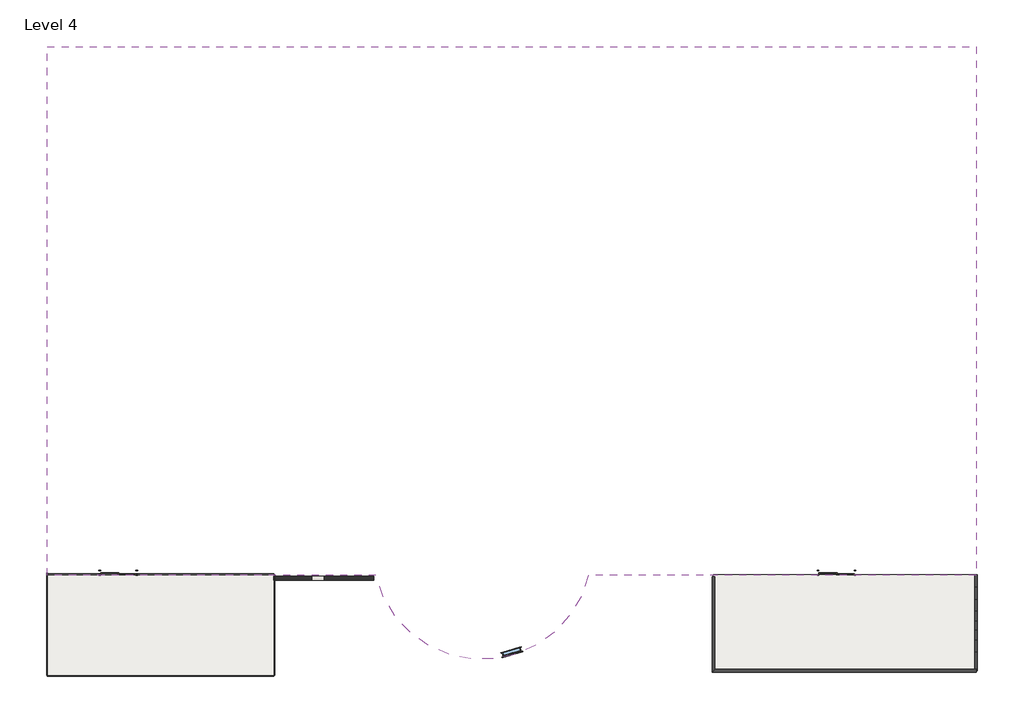
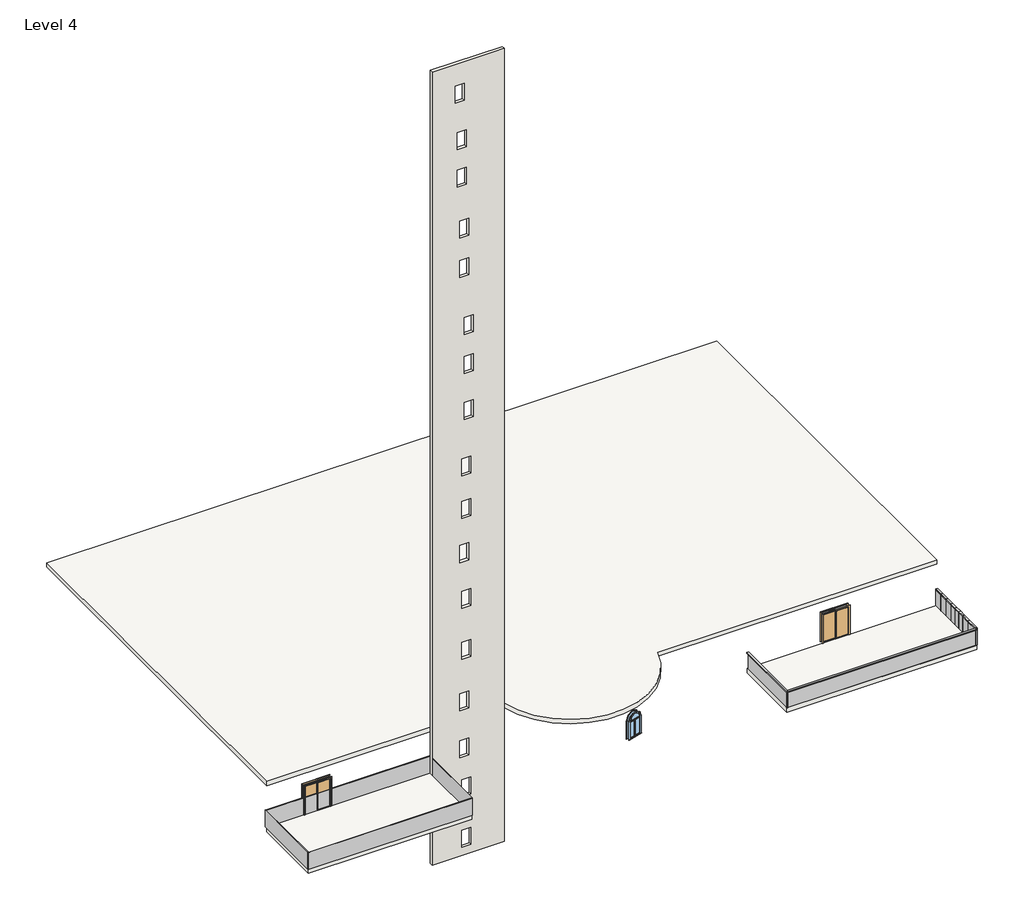
# One storey: 14 plates, 11 members, 3 slabs, 2 doors, 1 wall, 1 window.
"""IFC4 building model written with IfcOpenShell, lengths in millimetres."""

from ifc_helpers import new_model, si_unit, point, frame, frame_2d, origin, place, context, project, spatial, polyline, circle_curve, trimmed, segment, composite_curve, outline, extrude, transform, mapped, element, save
from components import door_076b30e0, member_75074519, member_47bfaf8a, member_15823cb3, member_e44847c7, member_d2e7e466, member_2fad0b47, member_fc190105, system_panel_glazed_7af1c9c3, system_panel_glazed_a18a7e0a, system_panel_glazed_7cd9bc56, system_panel_glazed_88916357, system_panel_glazed_11b37e3b, system_panel_glazed_6b3781c5, system_panel_glazed_3a47dc32, system_panel_glazed_b96adab1, system_panel_glazed_dcca9b78, window_cf4adaea

model = new_model("IFC4")

# Units and contexts
model_context = context("Model", 3, world=origin())
ifc_project = project(units=[si_unit("LENGTHUNIT", "METRE", prefix="MILLI")], contexts=[model_context])

# Site, building, storey
site = spatial("IfcSite", under=ifc_project)
building = spatial("IfcBuilding", under=site)
storey = spatial("IfcBuildingStorey", under=building, Name="Level 4", Elevation=6400.8)

# Doors
placement = place(None, origin())
door_shape = door_076b30e0(model_context)
element("IfcDoor", 1, ObjectType="Door-Double-Sliding : 68\" x 80\"", at=placement, inside=storey, context=model_context, shape_type="MappedRepresentation", body=[
    mapped(door_shape, transform((-16369.385279, -12227.7237084, 6400.8), x_axis=(-1.0, 0.0, 0.0), y_axis=(0.0, -1.0, 0.0), z_axis=(0.0, 0.0, 1.0))),
])
element("IfcDoor", 2, ObjectType="Door-Double-Sliding : 68\" x 80\"", at=placement, inside=storey, context=model_context, shape_type="MappedRepresentation", body=[
    mapped(door_shape, transform((18682.614721, -12227.7237084, 6400.8), x_axis=(-1.0, 0.0, 0.0), y_axis=(0.0, -1.0, 0.0), z_axis=(0.0, 0.0, 1.0))),
])

# Members
member_shape = member_75074519(model_context)
element("IfcMember", 3, ObjectType="Rectangular Mullion : 2.5\" x 5\" rectangular", at=placement, inside=storey, context=model_context, shape_type="MappedRepresentation", body=[
    mapped(member_shape, transform((25489.814721, -17133.9605259, 7620.0), x_axis=(0.0, -1.0, 0.0), y_axis=(1.0, 0.0, 0.0), z_axis=(0.0, 0.0, 1.0))),
])
member_2_shape = member_47bfaf8a(model_context)
element("IfcMember", 4, ObjectType="Rectangular Mullion : 2.5\" x 5\" rectangular", at=placement, inside=storey, context=model_context, shape_type="MappedRepresentation", body=[
    mapped(member_2_shape, transform((25489.814721, -15609.9605259, 7620.0), x_axis=(0.0, 0.0, 1.0), y_axis=(1.0, 0.0, 0.0), z_axis=(0.0, 1.0, 0.0))),
])
member_3_shape = member_15823cb3(model_context)
element("IfcMember", 5, ObjectType="Rectangular Mullion : 2.5\" x 5\" rectangular", at=placement, inside=storey, context=model_context, shape_type="MappedRepresentation", body=[
    mapped(member_3_shape, transform((25489.814721, -14238.3605259, 7620.0), x_axis=(0.0, 0.0, 1.0), y_axis=(1.0, 0.0, 0.0), z_axis=(0.0, 1.0, 0.0))),
])
element("IfcMember", 6, ObjectType="Rectangular Mullion : 2.5\" x 5\" rectangular", at=placement, inside=storey, context=model_context, shape_type="MappedRepresentation", body=[
    mapped(member_3_shape, transform((25489.814721, -14695.5605259, 7620.0), x_axis=(0.0, 0.0, 1.0), y_axis=(1.0, 0.0, 0.0), z_axis=(0.0, 1.0, 0.0))),
])
element("IfcMember", 7, ObjectType="Rectangular Mullion : 2.5\" x 5\" rectangular", at=placement, inside=storey, context=model_context, shape_type="MappedRepresentation", body=[
    mapped(member_3_shape, transform((25489.814721, -15152.7605259, 7620.0), x_axis=(0.0, 0.0, 1.0), y_axis=(1.0, 0.0, 0.0), z_axis=(0.0, 1.0, 0.0))),
])
member_4_shape = member_e44847c7(model_context)
element("IfcMember", 8, ObjectType="Rectangular Mullion : 2.5\" x 5\" rectangular", at=placement, inside=storey, context=model_context, shape_type="MappedRepresentation", body=[
    mapped(member_4_shape, transform((25489.814721, -13050.3359809, 7620.0), x_axis=(0.0, 0.0, 1.0), y_axis=(1.0, 0.0, 0.0), z_axis=(0.0, 1.0, 0.0))),
])
element("IfcMember", 9, ObjectType="Rectangular Mullion : 2.5\" x 5\" rectangular", at=placement, inside=storey, context=model_context, shape_type="MappedRepresentation", body=[
    mapped(member_4_shape, transform((25489.814721, -13644.3482534, 7620.0), x_axis=(0.0, 0.0, 1.0), y_axis=(1.0, 0.0, 0.0), z_axis=(0.0, 1.0, 0.0))),
])
element("IfcMember", 10, ObjectType="Rectangular Mullion : 2.5\" x 5\" rectangular", at=placement, inside=storey, context=model_context, shape_type="MappedRepresentation", body=[
    mapped(member_4_shape, transform((25489.814721, -12456.3237084, 7620.0), x_axis=(0.0, 0.0, 1.0), y_axis=(1.0, 0.0, 0.0), z_axis=(0.0, 1.0, 0.0))),
])
member_5_shape = member_d2e7e466(model_context)
element("IfcMember", 11, ObjectType="Rectangular Mullion : 2.5\" x 5\" rectangular", at=placement, inside=storey, context=model_context, shape_type="MappedRepresentation", body=[
    mapped(member_5_shape, transform((25489.814721, -16219.5605259, 7620.0), x_axis=(0.0, 0.0, 1.0), y_axis=(1.0, 0.0, 0.0), z_axis=(0.0, 1.0, 0.0))),
])
member_6_shape = member_2fad0b47(model_context)
element("IfcMember", 12, ObjectType="Rectangular Mullion : 2.5\" x 5\" rectangular", at=placement, inside=storey, context=model_context, shape_type="MappedRepresentation", body=[
    mapped(member_6_shape, transform((12667.5594464, -17133.9605259, 7620.0), x_axis=(0.0, 0.0, 1.0), y_axis=(-1.0, 0.0, 0.0), z_axis=(0.0, -1.0, 0.0))),
])
member_7_shape = member_fc190105(model_context)
element("IfcMember", 13, ObjectType="Rectangular Mullion : 2.5\" x 5\" rectangular", at=placement, inside=storey, context=model_context, shape_type="MappedRepresentation", body=[
    mapped(member_7_shape, transform((25489.814721, -17133.9605259, 7620.0), x_axis=(0.0, 0.0, 1.0), y_axis=(0.0, -1.0, 0.0), z_axis=(1.0, 0.0, 0.0))),
])

# Plates
system_panel_glazed_shape = system_panel_glazed_7af1c9c3(model_context)
element("IfcPlate", 14, ObjectType="System Panel : Glazed", at=placement, inside=storey, context=model_context, shape_type="MappedRepresentation", body=[
    mapped(system_panel_glazed_shape, transform((25489.814721, -15914.7605259, 6400.8), x_axis=(0.0, 1.0, 0.0), y_axis=(-1.0, 0.0, 0.0), z_axis=(0.0, 0.0, 1.0))),
])
system_panel_glazed_2_shape = system_panel_glazed_a18a7e0a(model_context)
element("IfcPlate", 15, ObjectType="System Panel : Glazed", at=placement, inside=storey, context=model_context, shape_type="MappedRepresentation", body=[
    mapped(system_panel_glazed_2_shape, transform((25489.814721, -15381.3605259, 6400.8), x_axis=(0.0, 1.0, 0.0), y_axis=(-1.0, 0.0, 0.0), z_axis=(0.0, 0.0, 1.0))),
])
element("IfcPlate", 16, ObjectType="System Panel : Glazed", at=placement, inside=storey, context=model_context, shape_type="MappedRepresentation", body=[
    mapped(system_panel_glazed_2_shape, transform((25489.814721, -14924.1605259, 6400.8), x_axis=(0.0, 1.0, 0.0), y_axis=(-1.0, 0.0, 0.0), z_axis=(0.0, 0.0, 1.0))),
])
element("IfcPlate", 17, ObjectType="System Panel : Glazed", at=placement, inside=storey, context=model_context, shape_type="MappedRepresentation", body=[
    mapped(system_panel_glazed_2_shape, transform((25489.814721, -14466.9605259, 6400.8), x_axis=(0.0, 1.0, 0.0), y_axis=(-1.0, 0.0, 0.0), z_axis=(0.0, 0.0, 1.0))),
])
system_panel_glazed_3_shape = system_panel_glazed_7cd9bc56(model_context)
element("IfcPlate", 18, ObjectType="System Panel : Glazed", at=placement, inside=storey, context=model_context, shape_type="MappedRepresentation", body=[
    mapped(system_panel_glazed_3_shape, transform((19078.6870837, -17133.9605259, 6400.8), x_axis=(1.0, 0.0, 0.0), y_axis=(0.0, 1.0, 0.0), z_axis=(0.0, 0.0, 1.0))),
])
system_panel_glazed_4_shape = system_panel_glazed_88916357(model_context)
element("IfcPlate", 19, ObjectType="System Panel : Glazed", at=placement, inside=storey, context=model_context, shape_type="MappedRepresentation", body=[
    mapped(system_panel_glazed_4_shape, transform((25489.814721, -13941.3543897, 6400.8), x_axis=(0.0, 1.0, 0.0), y_axis=(-1.0, 0.0, 0.0), z_axis=(0.0, 0.0, 1.0))),
])
element("IfcPlate", 20, ObjectType="System Panel : Glazed", at=placement, inside=storey, context=model_context, shape_type="MappedRepresentation", body=[
    mapped(system_panel_glazed_4_shape, transform((25489.814721, -13347.3421172, 6400.8), x_axis=(0.0, 1.0, 0.0), y_axis=(-1.0, 0.0, 0.0), z_axis=(0.0, 0.0, 1.0))),
])
element("IfcPlate", 21, ObjectType="System Panel : Glazed", at=placement, inside=storey, context=model_context, shape_type="MappedRepresentation", body=[
    mapped(system_panel_glazed_4_shape, transform((25489.814721, -12753.3298446, 6400.8), x_axis=(0.0, 1.0, 0.0), y_axis=(-1.0, 0.0, 0.0), z_axis=(0.0, 0.0, 1.0))),
])
system_panel_glazed_5_shape = system_panel_glazed_11b37e3b(model_context)
element("IfcPlate", 22, ObjectType="System Panel : Glazed", at=placement, inside=storey, context=model_context, shape_type="MappedRepresentation", body=[
    mapped(system_panel_glazed_5_shape, transform((25489.814721, -16645.0105259, 6400.8), x_axis=(0.0, 1.0, 0.0), y_axis=(-1.0, 0.0, 0.0), z_axis=(0.0, 0.0, 1.0))),
])
system_panel_glazed_6_shape = system_panel_glazed_6b3781c5(model_context)
element("IfcPlate", 23, ObjectType="System Panel : Glazed", at=placement, inside=storey, context=model_context, shape_type="MappedRepresentation", body=[
    mapped(system_panel_glazed_6_shape, transform((12667.5594464, -14845.9421172, 6400.8), x_axis=(0.0, -1.0, 0.0), y_axis=(1.0, 0.0, 0.0), z_axis=(0.0, 0.0, 1.0))),
])
system_panel_glazed_7_shape = system_panel_glazed_3a47dc32(model_context)
element("IfcPlate", 24, ObjectType="System Panel : Glazed", at=placement, inside=storey, context=model_context, shape_type="MappedRepresentation", body=[
    mapped(system_panel_glazed_7_shape, transform((-8781.8000285, -14908.1863127, 6400.8), x_axis=(0.0, -1.0, 0.0), y_axis=(1.0, 0.0, 0.0), z_axis=(0.0, 0.0, 1.0))),
])
system_panel_glazed_8_shape = system_panel_glazed_b96adab1(model_context)
element("IfcPlate", 25, ObjectType="System Panel : Glazed", at=placement, inside=storey, context=model_context, shape_type="MappedRepresentation", body=[
    mapped(system_panel_glazed_8_shape, transform((-14302.7926538, -12456.3237084, 6400.8), x_axis=(1.0, 0.0, 0.0), y_axis=(0.0, 1.0, 0.0), z_axis=(0.0, 0.0, 1.0))),
])
element("IfcPlate", 26, ObjectType="System Panel : Glazed", at=placement, inside=storey, context=model_context, shape_type="MappedRepresentation", body=[
    mapped(system_panel_glazed_8_shape, transform((-14302.7926538, -17360.0489171, 6400.8), x_axis=(-1.0, 0.0, 0.0), y_axis=(0.0, -1.0, 0.0), z_axis=(0.0, 0.0, 1.0))),
])
system_panel_glazed_9_shape = system_panel_glazed_dcca9b78(model_context)
element("IfcPlate", 27, ObjectType="System Panel : Glazed", at=placement, inside=storey, context=model_context, shape_type="MappedRepresentation", body=[
    mapped(system_panel_glazed_9_shape, transform((-19823.785279, -14857.3863127, 6400.8), x_axis=(0.0, 1.0, 0.0), y_axis=(-1.0, 0.0, 0.0), z_axis=(0.0, 0.0, 1.0))),
])

# Slabs
element("IfcSlab", 28, ObjectType="Generic - 12\"", at=placement, inside=storey, context=model_context, shape_type="SweptSolid", body=[
    extrude(outline(composite_curve([segment(polyline([(25489.814721, 13322.6839017), (25489.814721, -12483.7160983), (6571.5594464, -12483.7160983)]), True, "CONTINUOUS"), segment(trimmed(circle_curve(frame_2d((1385.214721, -11253.083057)), 5330.3498284), [point((6571.5594464, -12483.7160983))], [point((-3801.1300045, -12483.7160983))], False, "CARTESIAN"), True, "CONTINUOUS"), segment(polyline([(-3801.1300045, -12483.7160983), (-19823.785279, -12483.7160983), (-19823.785279, 13322.6839017), (25489.814721, 13322.6839017)]), True, "CONTINUOUS")], self_intersect=False)), frame((0.0, 0.0, 9397.8634343), z_axis=(0.0, 0.0, 1.0), x_axis=(1.0, 0.0, 0.0)), (0.0, 0.0, 1.0), 304.8),
])
element("IfcSlab", 29, ObjectType="Generic - 12\"", at=placement, inside=storey, context=model_context, shape_type="SweptSolid", body=[
    extrude(outline(polyline([(25489.814721, -12456.3237084), (25489.814721, -17133.9605259), (12667.5594464, -17133.9605259), (12667.5594464, -12456.3237084), (25489.814721, -12456.3237084)])), frame((0.0, 0.0, 6096.0), z_axis=(0.0, 0.0, 1.0), x_axis=(1.0, 0.0, 0.0)), (0.0, 0.0, 1.0), 304.8),
])
element("IfcSlab", 30, ObjectType="Generic - 12\"", at=placement, inside=storey, context=model_context, shape_type="SweptSolid", body=[
    extrude(outline(polyline([(-8781.8000285, -12456.3237084), (-8781.8000285, -17360.0489171), (-19823.785279, -17360.0489171), (-19823.785279, -12456.3237084), (-8781.8000285, -12456.3237084)])), frame((0.0, 0.0, 6096.0), z_axis=(0.0, 0.0, 1.0), x_axis=(1.0, 0.0, 0.0)), (0.0, 0.0, 1.0), 304.8),
])

# Wall
element("IfcWall", 31, ObjectType="Generic - 8\"", at=placement, inside=storey, context=model_context, shape_type="SweptSolid", body=[
    extrude(outline(polyline([(0.0, -3905.0000285), (56730.1367162, -3905.0000285), (56730.1367162, -8781.8000285), (0.0, -8781.8000285), (0.0, -3905.0000285)]), holes=[polyline([(55168.8, -6615.785279), (53949.6, -6615.785279), (53949.6, -7225.385279), (55168.8, -7225.385279), (55168.8, -6615.785279)]), polyline([(51816.0, -6463.385279), (50596.8, -6463.385279), (50596.8, -7072.985279), (51816.0, -7072.985279), (51816.0, -6463.385279)]), polyline([(49118.1223994, -6463.385279), (47898.9223994, -6463.385279), (47898.9223994, -7072.985279), (49118.1223994, -7072.985279), (49118.1223994, -6463.385279)]), polyline([(45415.2, -6310.985279), (44196.0, -6310.985279), (44196.0, -6920.585279), (45415.2, -6920.585279), (45415.2, -6310.985279)]), polyline([(42596.9711489, -6310.985279), (41377.7711489, -6310.985279), (41377.7711489, -6920.585279), (42596.9711489, -6920.585279), (42596.9711489, -6310.985279)]), polyline([(38404.8, -6006.185279), (37185.6, -6006.185279), (37185.6, -6615.785279), (38404.8, -6615.785279), (38404.8, -6006.185279)]), polyline([(35612.9632624, -6006.185279), (34393.7632624, -6006.185279), (34393.7632624, -6615.785279), (35612.9632624, -6615.785279), (35612.9632624, -6006.185279)]), polyline([(32319.4939938, -6006.185279), (31100.2939938, -6006.185279), (31100.2939938, -6615.785279), (32319.4939938, -6615.785279), (32319.4939938, -6006.185279)]), polyline([(28346.4, -6158.585279), (27127.2, -6158.585279), (27127.2, -6768.185279), (28346.4, -6768.185279), (28346.4, -6158.585279)]), polyline([(25298.4, -6158.585279), (24079.2, -6158.585279), (24079.2, -6768.185279), (25298.4, -6768.185279), (25298.4, -6158.585279)]), polyline([(22198.213139, -6310.985279), (20979.013139, -6310.985279), (20979.013139, -6920.585279), (22198.213139, -6920.585279), (22198.213139, -6310.985279)]), polyline([(18878.7066858, -6158.585279), (17659.5066858, -6158.585279), (17659.5066858, -6768.185279), (18878.7066858, -6768.185279), (18878.7066858, -6158.585279)]), polyline([(15240.0, -6158.585279), (14020.8, -6158.585279), (14020.8, -6768.185279), (15240.0, -6768.185279), (15240.0, -6158.585279)]), polyline([(11582.4, -6310.985279), (10363.2, -6310.985279), (10363.2, -6920.585279), (11582.4, -6920.585279), (11582.4, -6310.985279)]), polyline([(8229.6, -6310.985279), (7010.4, -6310.985279), (7010.4, -6920.585279), (8229.6, -6920.585279), (8229.6, -6310.985279)]), polyline([(5394.6709372, -6158.585279), (4175.4709372, -6158.585279), (4175.4709372, -6768.185279), (5394.6709372, -6768.185279), (5394.6709372, -6158.585279)]), polyline([(1787.2275158, -6158.585279), (568.0275158, -6158.585279), (568.0275158, -6768.185279), (1787.2275158, -6768.185279), (1787.2275158, -6158.585279)])]), frame((0.0, -12718.8007309, 0.0), z_axis=(0.0, 1.0, 0.0), x_axis=(0.0, 0.0, 1.0)), (0.0, 0.0, 1.0), 203.2),
])

# Window
window_shape = window_cf4adaea(model_context)
element("IfcWindow", 32, ObjectType="36\" x 48\"", at=placement, inside=storey, context=model_context, shape_type="MappedRepresentation", body=[
    mapped(window_shape, transform((2839.5240885, -16227.6735606, 6400.8), x_axis=(-0.9606648902521716, -0.27771022422082875, 0.0), y_axis=(0.27771022422082875, -0.9606648902521716, 0.0), z_axis=(0.0, 0.0, 1.0))),
])

save(model, "model.ifc")

# Revit data of these elements
# Type "Door-Double-Sliding : 68\" x 80\""
#   Type Mark = "10"
#   Construction Type Id = "opn-d45"
#   Assembly Code = "C1020"
#   Analytic Construction = "Wood frame, double glass door "
#   Thickness = 0' - 2"
#   Thermal Resistance (R) = 1.8150 (h·ft²·°F)/BTU
#   Heat Transfer Coefficient (U) = 0.5510 BTU/(h·ft²·°F)
#   Height = 6' - 8"
#   Rail Width = 0' - 2"
#   Stiles = 0' - 2"
#   Trim Projection Ext = 0' - 1"
#   Trim Projection Int = 0' - 1"
#   Trim Width = 0' - 3"
#   Width = 5' - 8"
#   Define Thermal Properties by = 1
#   Glazing = Glass
#   Panel Material = Wood - Birch - Solid Stained Light Low Gloss
#   Trim Material = Paint - Sienna
#   Visual Light Transmittance = 0
#   Solar Heat Gain Coefficient = 0
#   Function = (empty or 0)
#   Wall Closure = (empty or 0)
# Type "Rectangular Mullion : 2.5\" x 5\" rectangular"
#   built-in parameter 1007304 = 0.416667 (stored number, unit not read)
#   built-in parameter 1007301 = 0.104167 (stored number, unit not read)
#   built-in parameter 1007300 = 0.104167 (stored number, unit not read)
# Type "System Panel : Glazed"
#   Construction Type Id = "GSP4R"
#   Analytic Construction = "1/8 in Pilkington single glazing"
#   Visual Light Transmittance = 0.9
#   Solar Heat Gain Coefficient = 0.86
#   Heat Transfer Coefficient (U) = 1.18115 BTU/(h·ft²·°F)
# Type "Generic - 12\""
#   Assembly Code = "B1010"
#   Function = 0
#   Layers, outside or top first: 1' - 0" no material (function 1)
# Type "Generic - 8\""
#   Assembly Code = "B2010"
#   Layers, outside or top first: 0' - 8" no material (function 1)
# Type "36\" x 48\""
#   Type Mark = "38"
#   Construction Type Id = "SGL"
#   Assembly Code = "B2020100"
#   Analytic Construction = "Large single-glazed windows"
#   Visual Light Transmittance = 0.9
#   Solar Heat Gain Coefficient = 0.86
#   Heat Transfer Coefficient (U) = 0.979472 BTU/(h·ft²·°F)
#   Height = 4' - 0"
#   Default Sill Height = 3' - 0"
#   Trim Projection - Ext. = 0' - 0 1/2"
#   Trim Projection - Int. = 0' - 0 3/4"
#   Trim Width - Exterior = 0' - 3 1/2"
#   Trim Width - Interior = 0' - 3 1/2"
#   Width = 3' - 0"
#   Window Inset = 0' - 0 3/4"
#   Define Thermal Properties by = 1
#   Glass Pane Material = Glass
#   Sash Material = Sash
#   Trim Exterior Material = Trim
#   Trim Interior Material = Trim
#   Wall Closure = (empty or 0)
# Elements 1, 2 (IfcDoor, "Door-Double-Sliding : 68\" x 80\"")
#   Phase Created = New Construction
#   Materials on its faces: "Paint - Sienna", "Wood - Birch - Solid Stained Light Low Gloss", "Glass"
# Elements 3, 4, 5, 6, 7, 8, 9, 10, 11, 12, 13 (IfcMember, "Rectangular Mullion : 2.5\" x 5\" rectangular")
#   Phase Created = New Construction
#   Materials on its faces: "Aluminum"
# Elements 14, 15, 16, 17, 18, 19, 20, 21, 22, 23, 24, 25, 26, 27 (IfcPlate, "System Panel : Glazed")
#   Phase Created = New Construction
#   Materials on its faces: "Glass"
# Element 28 (IfcSlab, "Generic - 12\"")
#   Height Offset From Level = 10' - 9.99462"
#   Phase Created = New Construction
#   Materials on its faces: "Default Floor"
# Elements 29, 30 (IfcSlab, "Generic - 12\"")
#   Height Offset From Level = 0' - 0"
#   Phase Created = New Construction
#   Materials on its faces: "Default Floor"
# Element 31 (IfcWall, "Generic - 8\"")
#   built-in parameter 1001111 = -21' - 0"
#   Top Offset = 0' - 0"
#   Base Offset = -21' - 0"
#   Unconnected Height = 186' - 1.46995"
#   wall height = 186' - 1.46995"
#   Phase Created = New Construction
#   Base Constraint = Level 4
#   Materials on its faces: "Default Wall"
# Element 32 (IfcWindow, "36\" x 48\"")
#   Mark = "32"
#   Phase Created = New Construction
#   Materials on its faces: "Sash", "Trim", "Glass"
# Materials
#   "Glass": class "Glass", colour RGB 0 128 192, transparency 0.75, Description = "Soda Lime Glass", Cost = 0
#   "Wood - Birch - Solid Stained Light Low Gloss": class "Wood", colour RGB 210 159 95, transparency 0, Cost = 0
#   "Paint - Sienna": colour RGB 118 70 51, transparency 0, Cost = 0
#   "Sash": class "Wood", colour RGB 224 178 126, transparency 0
#   "Trim": class "Wood", colour RGB 224 178 126, transparency 0
#   "Aluminum": class "Metal", colour RGB 247 247 247, transparency 0, Description = "Aluminum 6061", Cost = 0
#   "Default Floor": colour RGB 128 128 128, transparency 0
#   "Default Wall": colour RGB 128 128 128, transparency 0
